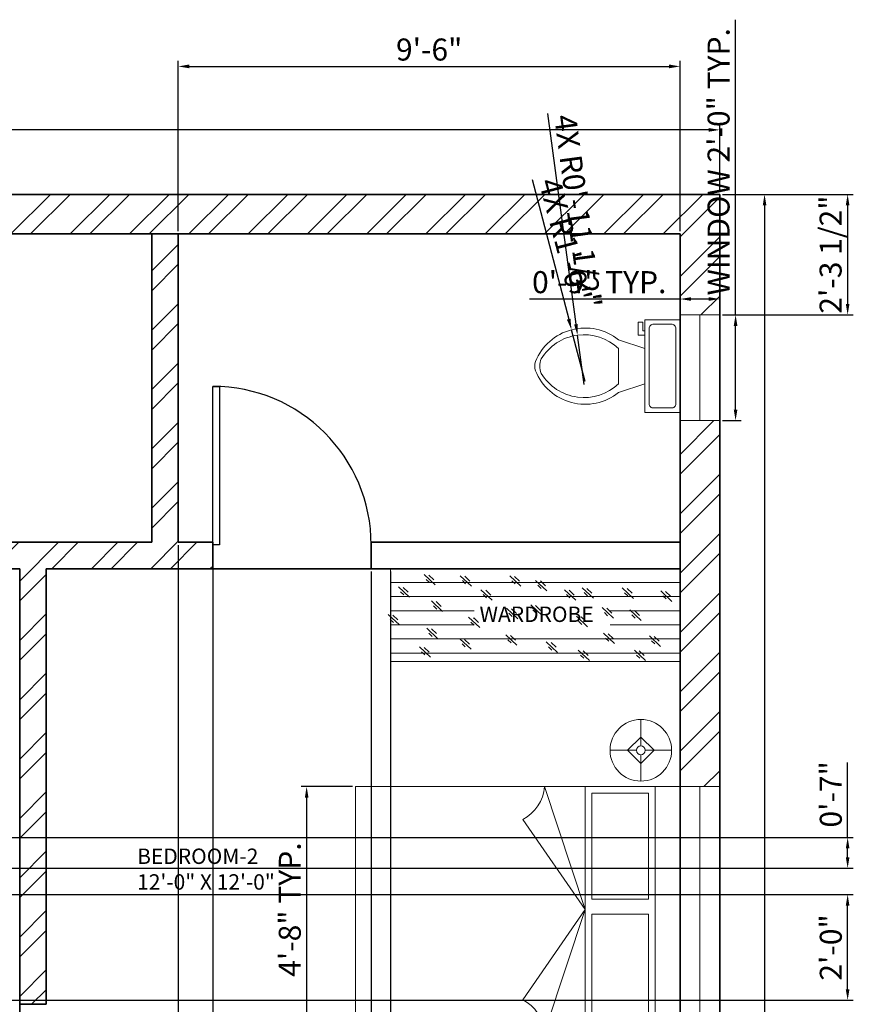
# Model space of a CAD drawing. Units: inches. Extents: x 28986 to 29505, y -162 to 451.
# Tile 6 of 6: x 29312 to 29504, y 228 to 451. Entities that reach past the tile are written whole.
import ezdxf

# ---------------------------------------------------------------- set-up
doc = ezdxf.new("R2010")
doc.units = ezdxf.units.IN
doc.layers.get('Defpoints').update_dxf_attribs({"color": 120})
for name, color, linetype, lineweight, true_color in [('A-ANNO-DIMS', 9, 'Continuous', 18, 0xafd9aa), ('A-FLOR-CASE', 32, 'Continuous', 18, 0xcd6928), ('A-FLOR-CASE-PATT', 32, 'Continuous', 13, 0xcd6928)]:
    doc.layers.add(name, color=color, linetype=linetype, lineweight=lineweight, true_color=true_color)
for name, color, linetype, lineweight in [('A-ANNO-TEXT', 6, 'Continuous', 18), ('A-AREA-IDEN', 6, 'Continuous', 18), ('A-FLOR-FIXT', 9, 'Continuous', 18), ('A-GLAZ', 4, 'Continuous', 18), ('A-WALL', 7, 'Continuous', 35), ('A-WALL-PATT', 1, 'Continuous', 13), ('DOOR', 2, 'Continuous', 25), ('FURNITURE', 241, 'Continuous', 18)]:
    doc.layers.add(name, color=color, linetype=linetype, lineweight=lineweight)
doc.styles.get("Standard").update_dxf_attribs({"font": 'arial.ttf'})
doc.dimstyles.new('ISO-25', dxfattribs={"dimtxt": 5, "dimasz": 2.5, "dimexe": 1.25, "dimexo": 0.625, "dimtad": 1, "dimdec": 0, "dimlunit": 3, "dimtxsty": 'Standard', "dimcen": 2.5, "dimadec": 0, "dimazin": 0, "dimtfac": 1, "dimtdec": 0, "dimtmove": 0, "dimatfit": 3, "dimfxl": 1, "dimarcsym": 0})

# ---------------------------------------------------------------- blocks, each defined once
blk = doc.blocks.new('*U4')
for p, q in [((0, 0), (0, -6)), ((40, 0), (40, -6))]:
    blk.add_line(p, q)
blk.add_lwpolyline([(0, 0), (0, 40), (1.75, 40), (1.75, 0)], close=True)
blk.add_arc((0, 0), 40, 0, 90)
blk = doc.blocks.new('modern bed')
for p, q in [((-55.85, 73.76), (-55.85, 0)), ((0, 0), (0, 73.76)), ((-55.85, 68.07), (0, 68.07)), ((-54.35, 66.57), (-54.35, 53.68)), ((-54.35, 66.57), (-30.33, 66.57)), ((-30.33, 66.57), (-30.33, 53.68)), ((-26.87, 66.57), (-1.5, 66.57)), ((-26.87, 66.57), (-26.87, 53.68)), ((-1.5, 53.68), (-1.5, 66.57)), ((-54.35, 53.68), (-30.33, 53.68)), ((-26.87, 53.68), (-1.5, 53.68)), ((-55.85, 52.18), (0, 52.18)), ((-27.93, 52.18), (-55.85, 42.95)), ((-27.93, 52.18), (-48.41, 38.03)), ((-27.93, 52.18), (0, 42.95)), ((-27.93, 52.18), (-7.44, 38.03)), ((-55.85, 0), (0, 0))]:
    blk.add_line(p, q)
blk.add_lwpolyline([(-55.85, 73.76), (0, 73.76)])
for centre, start, end in [((-56.5, 33.89), 27.0819, 85.9278), ((0.64, 33.89), 94.0722, 152.9181)]:
    blk.add_arc(centre, 9.08, start, end)
blk = doc.blocks.new('Lamp - Table')
for p, q in [((0, 7), (0, 1)), ((0, 3), (-3, 0)), ((3, 0), (0, 3)), ((-1, 0), (-7, 0)), ((-3, 0), (0, -3)), ((0, -3), (3, 0)), ((1, 0), (7, 0)), ((0, -1), (0, -7))]:
    blk.add_line(p, q)
for radius in [7, 1]:
    blk.add_circle((0, 0), radius)
blk = doc.blocks.new('Toilet - top')
for p, q in [((9.5, -6), (9.5, -2)), ((-10, -8.5), (-8, -8.5)), ((-10, -9.5), (-10, -8.5)), ((-8, -8.5), (-8, -8)), ((-7, -8), (-7, -9.5)), ((-4, -8), (-6, -14)), ((4, -8), (6, -14)), ((-7, -9.5), (-10, -9.5)), ((4, -14), (-4, -14))]:
    blk.add_line(p, q)
blk.add_lwpolyline([(10.5, -8), (10.5, 0), (-10.5, 0), (-10.5, -8)], close=True)
for points in [[(-9.5, -2), (-9.5, -6)], [(8.5, -1), (-8.5, -1)], [(-8.5, -7), (8.5, -7)]]:
    blk.add_lwpolyline(points)
for centre, radius, start, end in [((-8.62, -1.88), 0.884, 81.8699, 188.1301), ((8.62, -1.88), 0.884, 351.8699, 98.1301), ((-8.62, -6.12), 0.884, 171.8699, 278.1301), ((8.62, -6.12), 0.884, 261.8699, 8.1301), ((3.52, -21.58), 12.17, 141.4691, 247.9714), ((4.2, -21.82), 11.33, 136.3677, 238.9468), ((-3.52, -21.58), 12.17, 292.0284, 38.5307), ((-4.2, -21.82), 11.33, 301.053, 43.6321), ((0, -27.88), 4, 245.7318, 294.2682), ((0, -29), 4, 254.8605, 285.1395)]:
    blk.add_arc(centre, radius, start, end)
blk = doc.blocks.new('*D25')
at = {"layer": 'A-ANNO-DIMS', "color": 0, "lineweight": -2, "transparency": 16777216}
for p, q in [((29051.16, 412.32), (29051.16, 427.59)), ((29471.16, 412.32), (29471.16, 427.59)), ((29468.66, 426.34), (29053.66, 426.34))]:
    blk.add_line(p, q, dxfattribs=at)
at = {"layer": 'A-ANNO-DIMS', "color": 0, "transparency": 16777216}
for points in [[(29053.66, 426.75), (29053.66, 425.92), (29051.16, 426.34)], [(29468.66, 426.75), (29468.66, 425.92), (29471.16, 426.34)]]:
    blk.add_solid(points, dxfattribs=at)
at = {"layer": 'Defpoints', "color": 0, "transparency": 16777216}
for p in [(29051.16, 426.34), (29051.16, 411.7), (29471.16, 411.7)]:
    blk.add_point(p, dxfattribs=at)
at = {"layer": 'A-ANNO-DIMS', "color": 0, "transparency": 16777216, "insert": (29261.16, 429.52), "char_height": 5, "attachment_point": 5}
blk.add_mtext("35'", dxfattribs=at)
blk = doc.blocks.new('*D26')
at = {"layer": 'A-ANNO-DIMS', "color": 0, "lineweight": -2, "transparency": 16777216}
for p, q in [((29475.53, 411.7), (29482.59, 411.7)), ((29481.34, 409.2), (29481.34, -125.8)), ((29475.53, -128.3), (29482.59, -128.3))]:
    blk.add_line(p, q, dxfattribs=at)
at = {"layer": 'A-ANNO-DIMS', "color": 0, "transparency": 16777216}
for points in [[(29480.93, 409.2), (29481.76, 409.2), (29481.34, 411.7)], [(29480.93, -125.8), (29481.76, -125.8), (29481.34, -128.3)]]:
    blk.add_solid(points, dxfattribs=at)
at = {"layer": 'Defpoints', "color": 0, "transparency": 16777216}
for p in [(29474.91, 411.7), (29474.91, -128.3), (29481.34, -128.3)]:
    blk.add_point(p, dxfattribs=at)
at = {"layer": 'A-ANNO-DIMS', "color": 0, "transparency": 16777216, "insert": (29478.18, 141.7), "char_height": 5, "attachment_point": 5, "rotation": 90}
blk.add_mtext("45'", dxfattribs=at)
blk = doc.blocks.new('WIN-24IN')
for p, q in [((0, 0), (0, 9)), ((24, 0), (24, 9)), ((0, 4.5), (24, 4.5))]:
    blk.add_line(p, q)
blk = doc.blocks.new('WIN-55_85IN')
for p, q in [((0, 55.85), (9, 55.85)), ((4.5, 0), (4.5, 55.85)), ((0, 0), (9, 0))]:
    blk.add_line(p, q)
blk = doc.blocks.new('WARDROBE-REFLECTION-MARK')
for p, q in [((0, 2.38), (2.54, 0)), ((1.09, 2.24), (2.22, 1.16)), ((0.49, 1.26), (1.24, 0.54))]:
    blk.add_line(p, q)
blk = doc.blocks.new('*D34')
at = {"layer": 'A-ANNO-DIMS', "color": 0, "lineweight": -2, "transparency": 16777216}
for p, q in [((29387.77, 277.22), (29376.08, 277.22)), ((29377.33, 274.72), (29377.33, 223.87)), ((29387.77, 221.37), (29376.08, 221.37))]:
    blk.add_line(p, q, dxfattribs=at)
at = {"layer": 'A-ANNO-DIMS', "color": 0, "transparency": 16777216}
for points in [[(29376.92, 274.72), (29377.75, 274.72), (29377.33, 277.22)], [(29376.92, 223.87), (29377.75, 223.87), (29377.33, 221.37)]]:
    blk.add_solid(points, dxfattribs=at)
at = {"layer": 'Defpoints', "color": 0, "transparency": 16777216}
for p in [(29388.4, 277.22), (29377.33, 221.37), (29388.4, 221.37)]:
    blk.add_point(p, dxfattribs=at)
at = {"layer": 'A-ANNO-DIMS', "color": 0, "transparency": 16777216, "insert": (29374.15, 249.3), "char_height": 5, "attachment_point": 5, "rotation": 90}
blk.add_mtext('4\'-8" TYP.', dxfattribs=at)
blk = doc.blocks.new('*D39')
at = {"layer": 'A-ANNO-DIMS', "color": 0, "lineweight": -2, "transparency": 16777216}
for p, q in [((29474.76, 384.33), (29474.76, 451.35)), ((29471.78, 384.33), (29476.01, 384.33)), ((29474.76, 362.83), (29474.76, 381.83)), ((29471.78, 360.33), (29476.01, 360.33))]:
    blk.add_line(p, q, dxfattribs=at)
at = {"layer": 'A-ANNO-DIMS', "color": 0, "transparency": 16777216}
for points in [[(29474.34, 381.83), (29475.17, 381.83), (29474.76, 384.33)], [(29474.34, 362.83), (29475.17, 362.83), (29474.76, 360.33)]]:
    blk.add_solid(points, dxfattribs=at)
at = {"layer": 'Defpoints', "color": 0, "transparency": 16777216}
for p in [(29471.16, 384.33), (29474.76, 384.33), (29471.16, 360.33)]:
    blk.add_point(p, dxfattribs=at)
at = {"layer": 'A-ANNO-DIMS', "color": 0, "transparency": 16777216, "insert": (29471.54, 419.09), "char_height": 5, "attachment_point": 5, "rotation": 90}
blk.add_mtext('WINDOW 2\'-0" TYP.', dxfattribs=at)
blk = doc.blocks.new('*D40')
at = {"layer": 'A-ANNO-DIMS', "color": 0, "lineweight": -2, "transparency": 16777216}
for p, q in [((29462.16, 384.96), (29462.16, 389.18)), ((29471.16, 384.96), (29471.16, 389.18)), ((29462.16, 387.93), (29427.93, 387.93)), ((29468.66, 387.93), (29464.66, 387.93))]:
    blk.add_line(p, q, dxfattribs=at)
at = {"layer": 'A-ANNO-DIMS', "color": 0, "transparency": 16777216}
for points in [[(29464.66, 388.35), (29464.66, 387.52), (29462.16, 387.93)], [(29468.66, 388.35), (29468.66, 387.52), (29471.16, 387.93)]]:
    blk.add_solid(points, dxfattribs=at)
at = {"layer": 'Defpoints', "color": 0, "transparency": 16777216}
for p in [(29462.16, 387.93), (29462.16, 384.33), (29471.16, 384.33)]:
    blk.add_point(p, dxfattribs=at)
at = {"layer": 'A-ANNO-DIMS', "color": 0, "transparency": 16777216, "insert": (29443.79, 391.11), "char_height": 5, "attachment_point": 5}
blk.add_mtext('0\'-9" TYP.', dxfattribs=at)
blk = doc.blocks.new('*D63')
at = {"layer": 'A-ANNO-DIMS', "color": 0, "lineweight": -2, "transparency": 16777216}
for p, q in [((29348.16, 403.32), (29348.16, 442)), ((29350.66, 440.75), (29459.66, 440.75)), ((29462.16, 403.32), (29462.16, 442))]:
    blk.add_line(p, q, dxfattribs=at)
at = {"layer": 'A-ANNO-DIMS', "color": 0, "transparency": 16777216}
for points in [[(29350.66, 441.17), (29350.66, 440.33), (29348.16, 440.75)], [(29459.66, 441.17), (29459.66, 440.33), (29462.16, 440.75)]]:
    blk.add_solid(points, dxfattribs=at)
at = {"layer": 'Defpoints', "color": 0, "transparency": 16777216}
for p in [(29462.16, 440.75), (29348.16, 402.7), (29462.16, 402.7)]:
    blk.add_point(p, dxfattribs=at)
at = {"layer": 'A-ANNO-DIMS', "color": 0, "transparency": 16777216, "insert": (29405.16, 443.93), "char_height": 5, "attachment_point": 5}
blk.add_mtext('9\'-6"', dxfattribs=at)
blk = doc.blocks.new('*D67')
at = {"layer": 'A-ANNO-DIMS', "color": 0, "lineweight": -2, "transparency": 16777216}
for p, q in [((29471.78, 411.7), (29501.46, 411.7)), ((29500.21, 409.2), (29500.21, 386.83)), ((29471.78, 384.33), (29501.46, 384.33))]:
    blk.add_line(p, q, dxfattribs=at)
at = {"layer": 'A-ANNO-DIMS', "color": 0, "transparency": 16777216}
for points in [[(29499.79, 409.2), (29500.62, 409.2), (29500.21, 411.7)], [(29499.79, 386.83), (29500.62, 386.83), (29500.21, 384.33)]]:
    blk.add_solid(points, dxfattribs=at)
at = {"layer": 'Defpoints', "color": 0, "transparency": 16777216}
for p in [(29471.16, 411.7), (29471.16, 384.33), (29500.21, 384.33)]:
    blk.add_point(p, dxfattribs=at)
at = {"layer": 'A-ANNO-DIMS', "color": 0, "transparency": 16777216, "insert": (29496.99, 398.02), "char_height": 5, "attachment_point": 5, "rotation": 90}
blk.add_mtext('2\'-3 1/2"', dxfattribs=at)
blk = doc.blocks.new('*D79')
at = {"layer": 'A-ANNO-DIMS', "color": 0, "lineweight": -2, "transparency": 16777216}
for p, q in [((29355.99, 326.07), (29355.99, -158.6)), ((29391.99, 326.07), (29391.99, -158.6)), ((29358.49, -157.35), (29389.49, -157.35))]:
    blk.add_line(p, q, dxfattribs=at)
at = {"layer": 'A-ANNO-DIMS', "color": 0, "transparency": 16777216}
for points in [[(29358.49, -156.93), (29358.49, -157.77), (29355.99, -157.35)], [(29389.49, -156.93), (29389.49, -157.77), (29391.99, -157.35)]]:
    blk.add_solid(points, dxfattribs=at)
at = {"layer": 'Defpoints', "color": 0, "transparency": 16777216}
for p in [(29355.99, 326.7), (29391.99, 326.7), (29391.99, -157.35)]:
    blk.add_point(p, dxfattribs=at)
at = {"layer": 'A-ANNO-DIMS', "color": 0, "transparency": 16777216, "insert": (29373.99, -154.17), "char_height": 5, "attachment_point": 5}
blk.add_mtext('3\'-0"', dxfattribs=at)
blk = doc.blocks.new('*D80')
at = {"layer": 'A-ANNO-DIMS', "color": 0, "lineweight": -2, "transparency": 16777216}
for p, q in [((29348.16, 332.07), (29348.16, -158.6)), ((29355.99, 332.07), (29355.99, -158.6)), ((29350.66, -157.35), (29353.49, -157.35)), ((29355.99, -157.35), (29373.03, -157.35))]:
    blk.add_line(p, q, dxfattribs=at)
at = {"layer": 'A-ANNO-DIMS', "color": 0, "transparency": 16777216}
for points in [[(29350.66, -156.93), (29350.66, -157.77), (29348.16, -157.35)], [(29353.49, -156.93), (29353.49, -157.77), (29355.99, -157.35)]]:
    blk.add_solid(points, dxfattribs=at)
at = {"layer": 'Defpoints', "color": 0, "transparency": 16777216}
for p in [(29348.16, 332.7), (29355.99, 332.7), (29355.99, -157.35)]:
    blk.add_point(p, dxfattribs=at)
at = {"layer": 'A-ANNO-DIMS', "color": 0, "transparency": 16777216, "insert": (29365.76, -154.17), "char_height": 5, "attachment_point": 5}
blk.add_mtext('0\'-8"', dxfattribs=at)
blk = doc.blocks.new('*D85')
at = {"layer": 'A-ANNO-DIMS', "color": 0, "lineweight": -2, "transparency": 16777216}
for p, q in [((29500.21, 265.69), (29500.21, 282.73)), ((29204.78, 265.69), (29501.46, 265.69)), ((29500.21, 261.2), (29500.21, 263.19)), ((29204.78, 258.7), (29501.46, 258.7))]:
    blk.add_line(p, q, dxfattribs=at)
at = {"layer": 'A-ANNO-DIMS', "color": 0, "transparency": 16777216}
for points in [[(29499.79, 263.19), (29500.62, 263.19), (29500.21, 265.69)], [(29499.79, 261.2), (29500.62, 261.2), (29500.21, 258.7)]]:
    blk.add_solid(points, dxfattribs=at)
at = {"layer": 'Defpoints', "color": 0, "transparency": 16777216}
for p in [(29204.16, 265.69), (29500.21, 265.69), (29204.16, 258.7)]:
    blk.add_point(p, dxfattribs=at)
at = {"layer": 'A-ANNO-DIMS', "color": 0, "transparency": 16777216, "insert": (29497.03, 275.46), "char_height": 5, "attachment_point": 5, "rotation": 90}
blk.add_mtext('0\'-7"', dxfattribs=at)
blk = doc.blocks.new('*D96')
at = {"layer": 'A-ANNO-DIMS', "color": 0, "lineweight": -2, "transparency": 16777216}
for p, q in [((29391.99, 326.07), (29391.99, -158.6)), ((29396.38, 326.07), (29396.38, -158.6)), ((29389.49, -157.35), (29386.99, -157.35)), ((29391.99, -157.35), (29396.38, -157.35)), ((29398.88, -157.35), (29427.57, -157.35))]:
    blk.add_line(p, q, dxfattribs=at)
at = {"layer": 'A-ANNO-DIMS', "color": 0, "transparency": 16777216}
for points in [[(29389.49, -156.93), (29389.49, -157.77), (29391.99, -157.35)], [(29398.88, -156.93), (29398.88, -157.77), (29396.38, -157.35)]]:
    blk.add_solid(points, dxfattribs=at)
at = {"layer": 'Defpoints', "color": 0, "transparency": 16777216}
for p in [(29391.99, 326.7), (29396.38, 326.7), (29396.38, -157.35)]:
    blk.add_point(p, dxfattribs=at)
at = {"layer": 'A-ANNO-DIMS', "color": 0, "transparency": 16777216, "insert": (29414.48, -154.14), "char_height": 5, "attachment_point": 5}
blk.add_mtext('0\'-4 1/2"', dxfattribs=at)
blk = doc.blocks.new('*D97')
at = {"layer": 'A-ANNO-DIMS', "color": 0, "lineweight": -2, "transparency": 16777216}
for p, q in [((29180.78, 252.7), (29501.46, 252.7)), ((29500.21, 231.2), (29500.21, 250.2)), ((29180.78, 228.7), (29501.46, 228.7))]:
    blk.add_line(p, q, dxfattribs=at)
at = {"layer": 'A-ANNO-DIMS', "color": 0, "transparency": 16777216}
for points in [[(29499.79, 250.2), (29500.62, 250.2), (29500.21, 252.7)], [(29499.79, 231.2), (29500.62, 231.2), (29500.21, 228.7)]]:
    blk.add_solid(points, dxfattribs=at)
at = {"layer": 'Defpoints', "color": 0, "transparency": 16777216}
for p in [(29180.16, 252.7), (29500.21, 252.7), (29180.16, 228.7)]:
    blk.add_point(p, dxfattribs=at)
at = {"layer": 'A-ANNO-DIMS', "color": 0, "transparency": 16777216, "insert": (29497.03, 240.7), "char_height": 5, "attachment_point": 5, "rotation": 90}
blk.add_mtext('2\'-0"', dxfattribs=at)
blk = doc.blocks.new('*D101')
at = {"layer": 'A-ANNO-DIMS', "color": 0, "lineweight": -2, "transparency": 16777216}
for p, q in [((29428.53, 415.05), (29436.86, 383.36)), ((29440.58, 369.17), (29437.49, 380.94))]:
    blk.add_line(p, q, dxfattribs=at)
at = {"layer": 'A-ANNO-DIMS', "color": 0, "transparency": 16777216}
blk.add_solid([(29437.26, 383.46), (29436.45, 383.25), (29437.49, 380.94)], dxfattribs=at)
at = {"layer": 'Defpoints', "color": 0, "transparency": 16777216}
for p in [(29437.49, 380.94), (29440.58, 369.17)]:
    blk.add_point(p, dxfattribs=at)
at = {"layer": 'A-ANNO-DIMS', "color": 0, "transparency": 16777216, "insert": (29435.45, 401.22), "char_height": 5, "attachment_point": 5, "rotation": 284.7209}
blk.add_mtext('4X R1\'-0"', dxfattribs=at)
blk = doc.blocks.new('*D102')
at = {"layer": 'A-ANNO-DIMS', "color": 0, "lineweight": -2, "transparency": 16777216}
for p, q in [((29432.07, 430.07), (29438.5, 382.2)), ((29440.35, 368.49), (29438.84, 379.72))]:
    blk.add_line(p, q, dxfattribs=at)
at = {"layer": 'A-ANNO-DIMS', "color": 0, "transparency": 16777216}
blk.add_solid([(29438.92, 382.25), (29438.09, 382.14), (29438.84, 379.72)], dxfattribs=at)
at = {"layer": 'Defpoints', "color": 0, "transparency": 16777216}
for p in [(29438.84, 379.72), (29440.35, 368.49)]:
    blk.add_point(p, dxfattribs=at)
at = {"layer": 'A-ANNO-DIMS', "color": 0, "transparency": 16777216, "insert": (29438.3, 407.8), "char_height": 5, "attachment_point": 5, "rotation": 277.6562}
blk.add_mtext('4X R0\'-11 1/2"', dxfattribs=at)

msp = doc.modelspace()

# ---------------------------------------------------------------- hatches: boundary and pattern name
at = {"layer": 'A-WALL-PATT'}
h = msp.add_hatch(dxfattribs=at)
h.set_pattern_fill('ANSI32', color=256)
h.paths.add_polyline_path([(29174.16, 34.7), (29163.04, 34.7), (29163.04, 29.3), (29163.04, 25.7), (29168.16, 25.7), (29168.16, -119.3), (29174.16, -119.3), (29174.16, -71.3), (29199.96, -71.3), (29199.96, -65.3), (29174.16, -65.3)])
h.paths.add_polyline_path([(29244.8, -65.3), (29235.96, -65.3), (29235.96, -71.3), (29244.8, -71.3)])
h.paths.add_polyline_path([(29318.16, 39.7), (29462.16, 39.7), (29462.16, 44.7), (29318.16, 44.7), (29318.16, 131.49), (29312.16, 131.49), (29312.16, -65.3), (29292.8, -65.3), (29292.8, -71.3), (29312.16, -71.3), (29312.16, -119.3), (29318.16, -119.3)])
h.paths.add_polyline_path([(29219.6, 411.7), (29051.16, 411.7), (29051.16, 368.84), (29060.16, 368.84), (29060.16, 402.7), (29204.16, 402.7), (29219.6, 402.7)])
h.paths.add_polyline_path([(29060.16, 320.84), (29051.16, 320.84), (29051.16, 231.24), (29060.16, 231.24), (29060.16, 252.7)])
h.paths.add_polyline_path([(29210.16, 265.69), (29204.76, 265.69), (29204.16, 265.69), (29204.16, 258.7), (29060.16, 258.7), (29060.16, 252.7), (29204.16, 252.7), (29204.16, 228.7), (29204.16, 168.7), (29199.96, 168.7), (29199.96, 167.47), (29199.96, 162.7), (29210.16, 162.7)])
h.paths.add_polyline_path([(29060.16, 183.24), (29051.16, 183.24), (29051.16, 162.7), (29060.16, 162.7), (29168.16, 162.7), (29168.16, 167.47), (29168.16, 168.7), (29060.16, 168.7)])
h.paths.add_polyline_path([(29060.16, 126.7), (29051.16, 126.7), (29051.16, 70.7), (29060.16, 70.7)])
h.paths.add_polyline_path([(29060.16, 25.7), (29127.04, 25.7), (29127.04, 34.7), (29060.16, 34.7), (29051.16, 34.7), (29051.16, -22.45), (29060.16, -22.45)])
h.paths.add_polyline_path([(29060.16, -70.45), (29051.16, -70.45), (29051.16, -128.3), (29084.16, -128.3), (29084.16, -119.3), (29060.16, -119.3)])
h.paths.add_polyline_path([(29174.16, -119.3), (29168.16, -119.3), (29132.16, -119.3), (29132.16, -128.3), (29174.16, -128.3)])
h.paths.add_polyline_path([(29471.16, 79.78), (29462.16, 79.78), (29462.16, -119.3), (29462.16, -128.3), (29471.16, -128.3)])
h.paths.add_polyline_path([(29462.16, 182.7), (29318.16, 182.7), (29318.16, 191.79), (29317.56, 191.79), (29312.16, 191.79), (29312.16, 167.49), (29317.56, 167.49), (29318.16, 167.49), (29318.16, 176.7), (29462.16, 176.7)])
h.paths.add_polyline_path([(29471.16, 221.37), (29462.16, 221.37), (29462.16, 135.64), (29471.16, 135.64)])
h.paths.add_polyline_path([(29471.16, 360.33), (29462.16, 360.33), (29462.16, 277.22), (29471.16, 277.22)])
h.paths.add_polyline_path([(29471.16, 411.7), (29243.6, 411.7), (29243.6, 402.7), (29462.16, 402.7), (29462.16, 384.33), (29471.16, 384.33)])
h.paths.add_polyline_path([(29348.16, 402.7), (29342.16, 402.7), (29342.16, 332.7), (29308.66, 332.7), (29308.66, 326.7), (29312.16, 326.7), (29312.16, 227.79), (29318.16, 227.79), (29318.16, 326.7), (29355.99, 326.7), (29355.99, 332.7), (29348.16, 332.7)])
h.paths.add_polyline_path([(29210.16, 326.7), (29272.66, 326.7), (29272.66, 332.1), (29272.66, 332.7), (29210.16, 332.7), (29210.16, 402.7), (29204.16, 402.7), (29204.16, 316.6), (29204.16, 301.69), (29210.16, 301.69)])

# ---------------------------------------------------------------- linework, layer by layer
at = {"layer": 'A-FLOR-CASE'}
for p, q in [((29396.38, 326.7), (29396.38, 305.66)), ((29418.18, 317.62), (29420.73, 315.23))]:
    msp.add_line(p, q, dxfattribs=at)
msp.add_lwpolyline([(29396.38, 305.66), (29462.16, 305.66), (29462.16, 326.7), (29391.99, 326.7)], dxfattribs=at)
at = {"layer": 'A-WALL'}
for p, q in [((29471.16, 411.7), (29051.16, 411.7)), ((29471.16, -128.3), (29471.16, 411.7)), ((29462.16, 402.7), (29060.16, 402.7)), ((29342.16, 332.7), (29342.16, 402.7)), ((29348.16, 332.7), (29348.16, 402.7)), ((29462.16, -119.3), (29462.16, 402.7)), ((29342.16, 332.7), (29308.66, 332.7)), ((29355.99, 332.7), (29348.16, 332.7)), ((29355.99, 332.7), (29355.99, 326.7)), ((29462.16, 332.7), (29391.99, 332.7)), ((29391.99, 332.7), (29391.99, 326.7)), ((29312.16, 326.7), (29210.16, 326.7)), ((29312.16, 326.7), (29312.16, -65.3)), ((29318.16, 326.7), (29318.16, 227.79)), ((29391.99, 326.7), (29318.16, 326.7)), ((29462.16, 326.7), (29391.99, 326.7)), ((29318.16, 227.79), (29312.16, 227.79))]:
    msp.add_line(p, q, dxfattribs=at)

# ---------------------------------------------------------------- block references
at = {"layer": 'A-FLOR-CASE'}
for p in [(29403.99, 323.02), (29412.21, 322.73), (29423.46, 322.7), (29398.16, 320.22), (29429.33, 321.67), (29449.02, 319.97), (29457.77, 319.28), (29405.68, 316.99), (29395.85, 313.94), (29450.74, 314.95), (29404.61, 310.8), (29412.13, 308.4), (29422.54, 309.3), (29444.74, 309.68), (29455.17, 309.07), (29402.96, 306.58), (29431.77, 307.69), (29439.04, 305.83), (29451.79, 305.83)]:
    msp.add_blockref('WARDROBE-REFLECTION-MARK', p, dxfattribs=at)
at = {"layer": 'A-FLOR-FIXT', "rotation": 270}
msp.add_blockref('Toilet - top', (29462.16, 372.69), dxfattribs=at)
at = {"layer": 'A-GLAZ', "rotation": 89.99999999997524}
msp.add_blockref('WIN-24IN', (29471.16, 360.33), dxfattribs=at)
at = {"layer": 'A-GLAZ'}
msp.add_blockref('WIN-55_85IN', (29462.16, 221.37), dxfattribs=at)
at = {"layer": 'DOOR', "xscale": 0.8999999999999752, "yscale": 0.8999999999999752, "zscale": 0.8999999999999752}
msp.add_blockref('*U4', (29355.99, 332.1), dxfattribs=at)
at = {"layer": 'FURNITURE'}
msp.add_blockref('Lamp - Table', (29453.24, 285.47), dxfattribs=at)
at = {"layer": 'FURNITURE', "rotation": 270}
msp.add_blockref('modern bed', (29388.4, 221.37), dxfattribs=at)

# ---------------------------------------------------------------- texts
at = {"layer": 'A-AREA-IDEN', "insert": (29338.83, 263.16), "char_height": 3.5, "attachment_point": 1}
msp.add_mtext_dynamic_manual_height_columns('BEDROOM-2\\P12\'-0" X 12\'-0"', width=65.867, gutter_width=12.5, heights=[0], dxfattribs=at)

# ---------------------------------------------------------------- dimensions: what is measured, and where the dimension line sits
at = {"layer": 'A-ANNO-DIMS'}
for base, p1, p2, angle, text, picture, middle in [((29474.76, 384.33), (29471.16, 360.33), (29471.16, 384.33), 90, 'WINDOW <> TYP.', '*D39', (29471.54, 419.09)), ((29462.16, 387.93), (29471.16, 384.33), (29462.16, 384.33), 180, '<> TYP.', '*D40', (29443.79, 391.11)), ((29377.3318, 221.3714), (29388.396, 277.2231), (29388.396, 221.3714), 270, '<> TYP.', '*D34', (29374.154, 249.2972))]:
    dim = msp.add_linear_dim(base=base, p1=p1, p2=p2, angle=angle, text=text, dimstyle='ISO-25', override={"dimdec": 1, "dimlfac": 1, "dimrnd": 0, "dimzin": 1, "dimdsep": 46, "dimlunit": 4, "dimfrac": 2}, dxfattribs=at)
    dim.commit()
    dim.dimension.update_dxf_attribs({"geometry": picture, "text_midpoint": middle})
for base, p1, p2, override, picture, middle in [((29462.16, 440.75), (29348.16, 402.7), (29462.16, 402.7), {"dimdec": 1, "dimlfac": 1, "dimrnd": 0, "dimzin": 1, "dimdsep": 46, "dimlunit": 4, "dimfrac": 2}, '*D63', (29405.16, 443.93)), ((29051.16, 426.34), (29471.16, 411.7), (29051.16, 411.7), {"dimclrd": 0, "dimclre": 0, "dimclrt": 0}, '*D25', (29261.16, 429.52)), ((29355.99, -157.35), (29348.16, 332.7), (29355.99, 332.7), {"dimdec": 1, "dimlfac": 1, "dimrnd": 0, "dimzin": 1, "dimdsep": 46, "dimlunit": 4, "dimfrac": 2}, '*D80', (29365.76, -154.17)), ((29391.99, -157.35), (29355.99, 326.7), (29391.99, 326.7), {"dimdec": 1, "dimlfac": 1, "dimrnd": 0, "dimzin": 1, "dimdsep": 46, "dimlunit": 4, "dimfrac": 2}, '*D79', (29373.99, -154.17))]:
    dim = msp.add_linear_dim(base=base, p1=p1, p2=p2, dimstyle='ISO-25', override=override, dxfattribs=at)
    dim.commit()
    dim.dimension.update_dxf_attribs({"geometry": picture, "text_midpoint": middle})
for center, mpoint, picture, middle in [((29440.35, 368.49), (29438.84, 379.72), '*D102', (29438.3, 407.8)), ((29440.58, 369.17), (29437.49, 380.94), '*D101', (29435.45, 401.22))]:
    dim = msp.add_radius_dim(center=center, mpoint=mpoint, text='4X <>', dimstyle='ISO-25', override={"dimdec": 1, "dimlfac": 1, "dimrnd": 0, "dimzin": 1, "dimdsep": 46, "dimlunit": 4, "dimfrac": 2}, dxfattribs=at)
    dim.commit()
    dim.dimension.update_dxf_attribs({"geometry": picture, "text_midpoint": middle})
for base, p1, p2, override, picture, middle in [((29500.21, 384.33), (29471.16, 411.7), (29471.16, 384.33), {"dimdec": 1, "dimlfac": 1, "dimrnd": 0, "dimzin": 1, "dimdsep": 46, "dimlunit": 4, "dimfrac": 2}, '*D67', (29496.99, 398.02)), ((29481.34, -128.3), (29474.91, 411.7), (29474.91, -128.3), {"dimclrd": 0, "dimclre": 0, "dimclrt": 0}, '*D26', (29478.18, 141.7)), ((29500.21, 265.69), (29204.16, 258.7), (29204.16, 265.69), {"dimdec": 1, "dimlfac": 1, "dimrnd": 0, "dimzin": 1, "dimdsep": 46, "dimlunit": 4, "dimfrac": 2}, '*D85', (29497.03, 275.46)), ((29500.21, 252.7), (29180.16, 228.7), (29180.16, 252.7), {"dimdec": 1, "dimlfac": 1, "dimrnd": 0, "dimzin": 1, "dimdsep": 46, "dimlunit": 4, "dimfrac": 2}, '*D97', (29497.03, 240.7))]:
    dim = msp.add_linear_dim(base=base, p1=p1, p2=p2, angle=90, dimstyle='ISO-25', override=override, dxfattribs=at)
    dim.commit()
    dim.dimension.update_dxf_attribs({"geometry": picture, "text_midpoint": middle})

# ---------------------------------------------------------------- next in the draw order: wipeouts: each hides what was drawn before it
msp.add_wipeout([(29415.37, 313.26), (29446.3, 313.26), (29446.3, 319.33), (29415.37, 319.33)]).dxf.layer = 'A-ANNO-TEXT'

# ---------------------------------------------------------------- next in the draw order: hatches: boundary and pattern name
at = {"layer": 'A-FLOR-CASE-PATT'}
h = msp.add_hatch(dxfattribs=at)
h.set_pattern_fill('ANSI31', color=256, scale=1.0089906, angle=-45, style=0)
h.paths.add_polyline_path([(29396.38, 305.66), (29462.16, 305.66), (29462.16, 326.7), (29396.38, 326.7)])
h.paths.add_polyline_path([(29415.37, 313.26), (29446.3, 313.26), (29446.3, 319.33), (29415.37, 319.33)], flags=0)

# ---------------------------------------------------------------- next in the draw order: block references
at = {"layer": 'A-FLOR-CASE'}
for p in [(29416.92, 319.55), (29435.9, 319.55), (29439.91, 320), (29422.76, 315.34), (29428.25, 316.08), (29444.46, 315.48), (29414.11, 313.32), (29438.59, 313.52)]:
    msp.add_blockref('WARDROBE-REFLECTION-MARK', p, dxfattribs=at)

# ---------------------------------------------------------------- next in the draw order: texts
at = {"layer": 'A-ANNO-TEXT', "insert": (29416.6, 318.1), "char_height": 3.5, "width": 65.867, "attachment_point": 1}
msp.add_mtext('WARDROBE', dxfattribs=at)

# ---------------------------------------------------------------- next in the draw order: dimensions: what is measured, and where the dimension line sits
at = {"layer": 'A-ANNO-DIMS'}
dim = msp.add_linear_dim(base=(29396.38, -157.35), p1=(29391.99, 326.7), p2=(29396.38, 326.7), dimstyle='ISO-25', override={"dimdec": 1, "dimlfac": 1, "dimrnd": 0, "dimzin": 1, "dimdsep": 46, "dimlunit": 4, "dimfrac": 2}, dxfattribs=at)
dim.commit()
dim.dimension.update_dxf_attribs({"geometry": '*D96', "text_midpoint": (29414.48, -154.14)})

doc.saveas('drawing.dxf')
